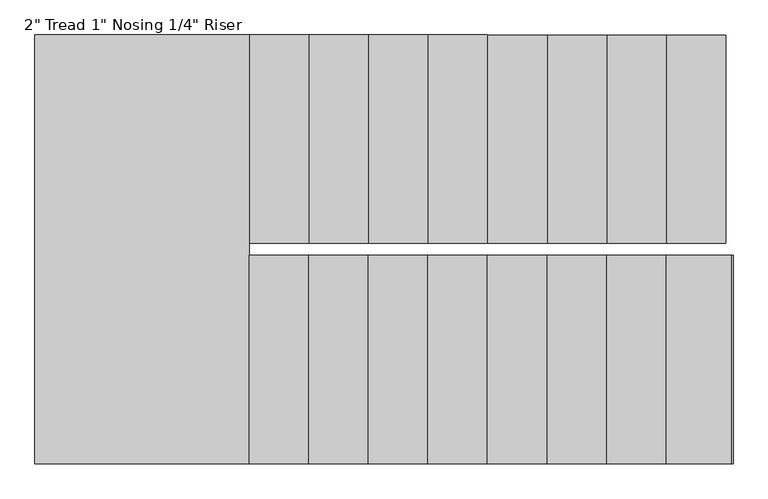
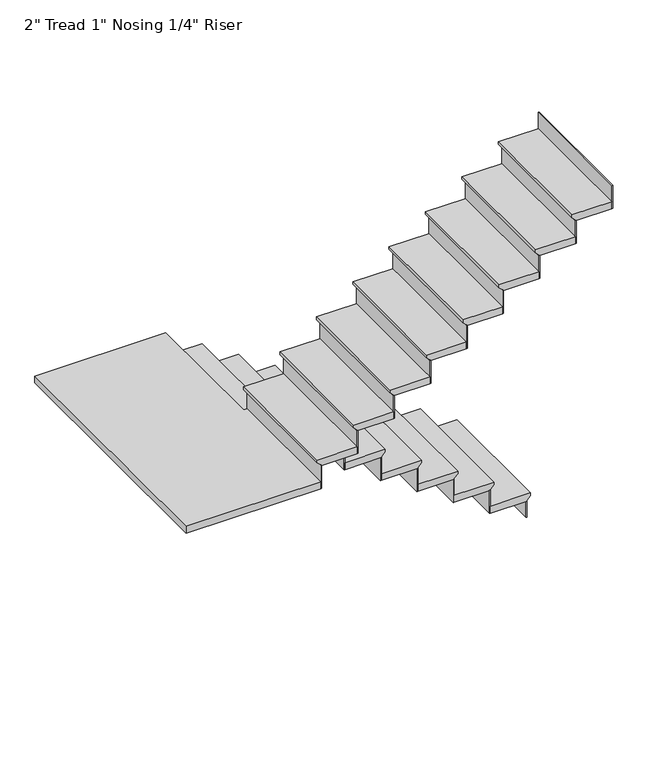
"""IFC4 building model written with IfcOpenShell, lengths in millimetres: stair flight geometry."""

from ifc_helpers import new_model, si_unit, origin, place, context, project, spatial, faceted_brep, source, transform, mapped, element, save


def stair_flight_02872950(model_context):
    return source(origin(), model_context, "Body", "Brep", [
        faceted_brep([(-2748.0012202, 5930.6309003, 6246.2833333), (-2748.0012202, 5930.6309003, 6265.3333333), (-2748.0012202, 5041.6309003, 6265.3333333), (-2748.0012202, 5041.6309003, 6246.2833333), (-2773.4012202, 5930.6309003, 6220.8833333), (-2773.4012202, 5041.6309003, 6220.8833333), (-3027.4012202, 5930.6309003, 6265.3333333), (-3027.4012202, 5041.6309003, 6265.3333333), (-2773.4012202, 5041.6309003, 6214.5333333), (-3027.4012202, 5041.6309003, 6214.5333333), (-3027.4012202, 5930.6309003, 6214.5333333), (-2773.4012202, 5930.6309003, 6214.5333333)], [[[0, 1, 2, 3]], [[4, 0, 3, 5]], [[2, 1, 6, 7]], [[8, 9, 10, 11]], [[2, 7, 9, 8, 5, 3]], [[8, 11, 4, 5]], [[6, 1, 0, 4, 11, 10]], [[7, 6, 10, 9]]]),
        faceted_brep([(-2773.4012202, 5930.6309003, 6214.5333333), (-2773.4012202, 5930.6309003, 6096.0), (-2779.7512202, 5930.6309003, 6096.0), (-2779.7512202, 5930.6309003, 6214.5333333), (-2773.4012202, 5041.6309003, 6214.5333333), (-2779.7512202, 5041.6309003, 6214.5333333), (-2779.7512202, 5041.6309003, 6096.0), (-2773.4012202, 5041.6309003, 6096.0)], [[[0, 1, 2, 3]], [[4, 5, 6, 7]], [[1, 0, 4, 7]], [[2, 1, 7, 6]], [[3, 2, 6, 5]], [[0, 3, 5, 4]]]),
        faceted_brep([(-3027.4012202, 5930.6309003, 6383.8666667), (-3027.4012202, 5930.6309003, 6214.5333333), (-3033.7512202, 5930.6309003, 6214.5333333), (-3033.7512202, 5930.6309003, 6383.8666667), (-3027.4012202, 5041.6309003, 6383.8666667), (-3033.7512202, 5041.6309003, 6383.8666667), (-3033.7512202, 5041.6309003, 6214.5333333), (-3027.4012202, 5041.6309003, 6214.5333333)], [[[0, 1, 2, 3]], [[4, 5, 6, 7]], [[1, 0, 4, 7]], [[2, 1, 7, 6]], [[3, 2, 6, 5]], [[0, 3, 5, 4]]]),
        faceted_brep([(-3002.0012202, 5041.6309003, 6434.6666667), (-3002.0012202, 5930.6309003, 6434.6666667), (-3281.4012202, 5930.6309003, 6434.6666667), (-3281.4012202, 5041.6309003, 6434.6666667), (-3027.4012202, 5041.6309003, 6383.8666667), (-3281.4012202, 5041.6309003, 6383.8666667), (-3281.4012202, 5930.6309003, 6383.8666667), (-3027.4012202, 5930.6309003, 6383.8666667), (-3027.4012202, 5041.6309003, 6390.2166667), (-3002.0012202, 5041.6309003, 6415.6166667), (-3027.4012202, 5930.6309003, 6390.2166667), (-3002.0012202, 5930.6309003, 6415.6166667)], [[[0, 1, 2, 3]], [[4, 5, 6, 7]], [[0, 3, 5, 4, 8, 9]], [[4, 7, 10, 8]], [[2, 1, 11, 10, 7, 6]], [[3, 2, 6, 5]], [[11, 1, 0, 9]], [[10, 11, 9, 8]]]),
        faceted_brep([(-3281.4012202, 5930.6309003, 6553.2), (-3281.4012202, 5930.6309003, 6383.8666667), (-3287.7512202, 5930.6309003, 6383.8666667), (-3287.7512202, 5930.6309003, 6553.2), (-3281.4012202, 5041.6309003, 6553.2), (-3287.7512202, 5041.6309003, 6553.2), (-3287.7512202, 5041.6309003, 6383.8666667), (-3281.4012202, 5041.6309003, 6383.8666667)], [[[0, 1, 2, 3]], [[4, 5, 6, 7]], [[1, 0, 4, 7]], [[2, 1, 7, 6]], [[3, 2, 6, 5]], [[0, 3, 5, 4]]]),
        faceted_brep([(-3256.0012202, 5041.6309003, 6604.0), (-3256.0012202, 5930.6309003, 6604.0), (-3535.4012202, 5930.6309003, 6604.0), (-3535.4012202, 5041.6309003, 6604.0), (-3281.4012202, 5041.6309003, 6553.2), (-3535.4012202, 5041.6309003, 6553.2), (-3535.4012202, 5930.6309003, 6553.2), (-3281.4012202, 5930.6309003, 6553.2), (-3281.4012202, 5041.6309003, 6559.55), (-3256.0012202, 5041.6309003, 6584.95), (-3281.4012202, 5930.6309003, 6559.55), (-3256.0012202, 5930.6309003, 6584.95)], [[[0, 1, 2, 3]], [[4, 5, 6, 7]], [[0, 3, 5, 4, 8, 9]], [[4, 7, 10, 8]], [[2, 1, 11, 10, 7, 6]], [[3, 2, 6, 5]], [[11, 1, 0, 9]], [[10, 11, 9, 8]]]),
        faceted_brep([(-3535.4012202, 5930.6309003, 6722.5333333), (-3535.4012202, 5930.6309003, 6553.2), (-3541.7512202, 5930.6309003, 6553.2), (-3541.7512202, 5930.6309003, 6722.5333333), (-3535.4012202, 5041.6309003, 6722.5333333), (-3541.7512202, 5041.6309003, 6722.5333333), (-3541.7512202, 5041.6309003, 6553.2), (-3535.4012202, 5041.6309003, 6553.2)], [[[0, 1, 2, 3]], [[4, 5, 6, 7]], [[1, 0, 4, 7]], [[2, 1, 7, 6]], [[3, 2, 6, 5]], [[0, 3, 5, 4]]]),
        faceted_brep([(-3510.0012202, 5041.6309003, 6773.3333333), (-3510.0012202, 5930.6309003, 6773.3333333), (-3789.4012202, 5930.6309003, 6773.3333333), (-3789.4012202, 5041.6309003, 6773.3333333), (-3535.4012202, 5041.6309003, 6722.5333333), (-3789.4012202, 5041.6309003, 6722.5333333), (-3789.4012202, 5930.6309003, 6722.5333333), (-3535.4012202, 5930.6309003, 6722.5333333), (-3535.4012202, 5041.6309003, 6728.8833333), (-3510.0012202, 5041.6309003, 6754.2833333), (-3535.4012202, 5930.6309003, 6728.8833333), (-3510.0012202, 5930.6309003, 6754.2833333)], [[[0, 1, 2, 3]], [[4, 5, 6, 7]], [[0, 3, 5, 4, 8, 9]], [[4, 7, 10, 8]], [[2, 1, 11, 10, 7, 6]], [[3, 2, 6, 5]], [[11, 1, 0, 9]], [[10, 11, 9, 8]]]),
        faceted_brep([(-3789.4012202, 5930.6309003, 6891.8666667), (-3789.4012202, 5930.6309003, 6722.5333333), (-3795.7512202, 5930.6309003, 6722.5333333), (-3795.7512202, 5930.6309003, 6891.8666667), (-3789.4012202, 5041.6309003, 6891.8666667), (-3795.7512202, 5041.6309003, 6891.8666667), (-3795.7512202, 5041.6309003, 6722.5333333), (-3789.4012202, 5041.6309003, 6722.5333333)], [[[0, 1, 2, 3]], [[4, 5, 6, 7]], [[1, 0, 4, 7]], [[2, 1, 7, 6]], [[3, 2, 6, 5]], [[0, 3, 5, 4]]]),
        faceted_brep([(-3764.0012202, 5041.6309003, 6942.6666667), (-3764.0012202, 5930.6309003, 6942.6666667), (-4043.4012202, 5930.6309003, 6942.6666667), (-4043.4012202, 5041.6309003, 6942.6666667), (-3789.4012202, 5041.6309003, 6891.8666667), (-4043.4012202, 5041.6309003, 6891.8666667), (-4043.4012202, 5930.6309003, 6891.8666667), (-3789.4012202, 5930.6309003, 6891.8666667), (-3789.4012202, 5041.6309003, 6898.2166667), (-3764.0012202, 5041.6309003, 6923.6166667), (-3789.4012202, 5930.6309003, 6898.2166667), (-3764.0012202, 5930.6309003, 6923.6166667)], [[[0, 1, 2, 3]], [[4, 5, 6, 7]], [[0, 3, 5, 4, 8, 9]], [[4, 7, 10, 8]], [[2, 1, 11, 10, 7, 6]], [[3, 2, 6, 5]], [[11, 1, 0, 9]], [[10, 11, 9, 8]]]),
        faceted_brep([(-4043.4012202, 5930.6309003, 7061.2), (-4043.4012202, 5930.6309003, 6891.8666667), (-4049.7512202, 5930.6309003, 6891.8666667), (-4049.7512202, 5930.6309003, 7061.2), (-4043.4012202, 5041.6309003, 7061.2), (-4049.7512202, 5041.6309003, 7061.2), (-4049.7512202, 5041.6309003, 6891.8666667), (-4043.4012202, 5041.6309003, 6891.8666667)], [[[0, 1, 2, 3]], [[4, 5, 6, 7]], [[1, 0, 4, 7]], [[2, 1, 7, 6]], [[3, 2, 6, 5]], [[0, 3, 5, 4]]]),
        faceted_brep([(-4018.0012202, 5041.6309003, 7112.0), (-4018.0012202, 5930.6309003, 7112.0), (-4297.4012202, 5930.6309003, 7112.0), (-4297.4012202, 5041.6309003, 7112.0), (-4043.4012202, 5041.6309003, 7061.2), (-4297.4012202, 5041.6309003, 7061.2), (-4297.4012202, 5930.6309003, 7061.2), (-4043.4012202, 5930.6309003, 7061.2), (-4043.4012202, 5041.6309003, 7067.55), (-4018.0012202, 5041.6309003, 7092.95), (-4043.4012202, 5930.6309003, 7067.55), (-4018.0012202, 5930.6309003, 7092.95)], [[[0, 1, 2, 3]], [[4, 5, 6, 7]], [[0, 3, 5, 4, 8, 9]], [[4, 7, 10, 8]], [[2, 1, 11, 10, 7, 6]], [[3, 2, 6, 5]], [[11, 1, 0, 9]], [[10, 11, 9, 8]]]),
        faceted_brep([(-4297.4012202, 5930.6309003, 7230.5333333), (-4297.4012202, 5930.6309003, 7061.2), (-4303.7512202, 5930.6309003, 7061.2), (-4303.7512202, 5930.6309003, 7230.5333333), (-4297.4012202, 5041.6309003, 7230.5333333), (-4303.7512202, 5041.6309003, 7230.5333333), (-4303.7512202, 5041.6309003, 7061.2), (-4297.4012202, 5041.6309003, 7061.2)], [[[0, 1, 2, 3]], [[4, 5, 6, 7]], [[1, 0, 4, 7]], [[2, 1, 7, 6]], [[3, 2, 6, 5]], [[0, 3, 5, 4]]]),
        faceted_brep([(-4272.0012202, 5041.6309003, 7281.3333333), (-4272.0012202, 5930.6309003, 7281.3333333), (-4551.4012202, 5930.6309003, 7281.3333333), (-4551.4012202, 5041.6309003, 7281.3333333), (-4297.4012202, 5041.6309003, 7230.5333333), (-4551.4012202, 5041.6309003, 7230.5333333), (-4551.4012202, 5930.6309003, 7230.5333333), (-4297.4012202, 5930.6309003, 7230.5333333), (-4297.4012202, 5041.6309003, 7236.8833333), (-4272.0012202, 5041.6309003, 7262.2833333), (-4297.4012202, 5930.6309003, 7236.8833333), (-4272.0012202, 5930.6309003, 7262.2833333)], [[[0, 1, 2, 3]], [[4, 5, 6, 7]], [[0, 3, 5, 4, 8, 9]], [[4, 7, 10, 8]], [[2, 1, 11, 10, 7, 6]], [[3, 2, 6, 5]], [[11, 1, 0, 9]], [[10, 11, 9, 8]]]),
        faceted_brep([(-4551.4012202, 5930.6309003, 7399.8666667), (-4551.4012202, 5930.6309003, 7230.5333333), (-4557.7512202, 5930.6309003, 7230.5333333), (-4557.7512202, 5930.6309003, 7399.8666667), (-4551.4012202, 5041.6309003, 7399.8666667), (-4557.7512202, 5041.6309003, 7399.8666667), (-4557.7512202, 5041.6309003, 7230.5333333), (-4551.4012202, 5041.6309003, 7230.5333333)], [[[0, 1, 2, 3]], [[4, 5, 6, 7]], [[1, 0, 4, 7]], [[2, 1, 7, 6]], [[3, 2, 6, 5]], [[0, 3, 5, 4]]]),
        faceted_brep([(-4526.0012202, 5041.6309003, 7450.6666667), (-4526.0012202, 5930.6309003, 7450.6666667), (-4805.4012202, 5930.6309003, 7450.6666667), (-4805.4012202, 5041.6309003, 7450.6666667), (-4551.4012202, 5041.6309003, 7399.8666667), (-4805.4012202, 5041.6309003, 7399.8666667), (-4805.4012202, 5930.6309003, 7399.8666667), (-4551.4012202, 5930.6309003, 7399.8666667), (-4551.4012202, 5041.6309003, 7406.2166667), (-4526.0012202, 5041.6309003, 7431.6166667), (-4551.4012202, 5930.6309003, 7406.2166667), (-4526.0012202, 5930.6309003, 7431.6166667)], [[[0, 1, 2, 3]], [[4, 5, 6, 7]], [[0, 3, 5, 4, 8, 9]], [[4, 7, 10, 8]], [[2, 1, 11, 10, 7, 6]], [[3, 2, 6, 5]], [[11, 1, 0, 9]], [[10, 11, 9, 8]]]),
        faceted_brep([(-4805.4012202, 5930.6309003, 7569.2), (-4805.4012202, 5930.6309003, 7399.8666667), (-4811.7512202, 5930.6309003, 7399.8666667), (-4811.7512202, 5930.6309003, 7569.2), (-4805.4012202, 5041.6309003, 7569.2), (-4811.7512202, 5041.6309003, 7569.2), (-4811.7512202, 5041.6309003, 7399.8666667), (-4805.4012202, 5041.6309003, 7399.8666667)], [[[0, 1, 2, 3]], [[4, 5, 6, 7]], [[1, 0, 4, 7]], [[2, 1, 7, 6]], [[3, 2, 6, 5]], [[0, 3, 5, 4]]]),
        faceted_brep([(-4754.6012202, 4990.8309003, 7620.0), (-4780.0012202, 4990.8309003, 7620.0), (-4780.0012202, 5930.6309003, 7620.0), (-5694.4012202, 5930.6309003, 7620.0), (-5694.4012202, 4101.8309003, 7620.0), (-4754.6012202, 4101.8309003, 7620.0), (-4780.0012202, 4990.8309003, 7569.2), (-4754.6012202, 4990.8309003, 7569.2), (-4754.6012202, 4101.8309003, 7569.2), (-5694.4012202, 4101.8309003, 7569.2), (-5694.4012202, 5930.6309003, 7569.2), (-4805.4012202, 5930.6309003, 7569.2), (-4805.4012202, 5041.6309003, 7569.2), (-4780.0012202, 5041.6309003, 7569.2), (-4780.0012202, 5041.6309003, 7600.95), (-4780.0012202, 5930.6309003, 7600.95), (-4805.4012202, 5041.6309003, 7575.55), (-4805.4012202, 5930.6309003, 7575.55)], [[[0, 1, 2, 3, 4, 5]], [[6, 7, 8, 9, 10, 11, 12, 13]], [[1, 0, 7, 6]], [[2, 1, 6, 13, 14, 15]], [[13, 12, 16, 14]], [[12, 11, 17, 16]], [[3, 2, 15, 17, 11, 10]], [[4, 3, 10, 9]], [[5, 4, 9, 8]], [[0, 5, 8, 7]], [[17, 15, 14, 16]]]),
        faceted_brep([(-4754.6012202, 4101.8309003, 7738.5333333), (-4754.6012202, 4101.8309003, 7569.2), (-4748.2512202, 4101.8309003, 7569.2), (-4748.2512202, 4101.8309003, 7738.5333333), (-4754.6012202, 4990.8309003, 7738.5333333), (-4748.2512202, 4990.8309003, 7738.5333333), (-4748.2512202, 4990.8309003, 7569.2), (-4754.6012202, 4990.8309003, 7569.2)], [[[0, 1, 2, 3]], [[4, 5, 6, 7]], [[1, 0, 4, 7]], [[2, 1, 7, 6]], [[3, 2, 6, 5]], [[0, 3, 5, 4]]]),
        faceted_brep([(-4780.0012202, 4990.8309003, 7789.3333333), (-4780.0012202, 4101.8309003, 7789.3333333), (-4500.6012202, 4101.8309003, 7789.3333333), (-4500.6012202, 4990.8309003, 7789.3333333), (-4754.6012202, 4990.8309003, 7738.5333333), (-4500.6012202, 4990.8309003, 7738.5333333), (-4500.6012202, 4101.8309003, 7738.5333333), (-4754.6012202, 4101.8309003, 7738.5333333), (-4754.6012202, 4990.8309003, 7744.8833333), (-4780.0012202, 4990.8309003, 7770.2833333), (-4754.6012202, 4101.8309003, 7744.8833333), (-4780.0012202, 4101.8309003, 7770.2833333)], [[[0, 1, 2, 3]], [[4, 5, 6, 7]], [[0, 3, 5, 4, 8, 9]], [[4, 7, 10, 8]], [[2, 1, 11, 10, 7, 6]], [[3, 2, 6, 5]], [[11, 1, 0, 9]], [[10, 11, 9, 8]]]),
        faceted_brep([(-4500.6012202, 4101.8309003, 7907.8666667), (-4500.6012202, 4101.8309003, 7738.5333333), (-4494.2512202, 4101.8309003, 7738.5333333), (-4494.2512202, 4101.8309003, 7907.8666667), (-4500.6012202, 4990.8309003, 7907.8666667), (-4494.2512202, 4990.8309003, 7907.8666667), (-4494.2512202, 4990.8309003, 7738.5333333), (-4500.6012202, 4990.8309003, 7738.5333333)], [[[0, 1, 2, 3]], [[4, 5, 6, 7]], [[1, 0, 4, 7]], [[2, 1, 7, 6]], [[3, 2, 6, 5]], [[0, 3, 5, 4]]]),
        faceted_brep([(-4526.0012202, 4990.8309003, 7958.6666667), (-4526.0012202, 4101.8309003, 7958.6666667), (-4246.6012202, 4101.8309003, 7958.6666667), (-4246.6012202, 4990.8309003, 7958.6666667), (-4500.6012202, 4990.8309003, 7907.8666667), (-4246.6012202, 4990.8309003, 7907.8666667), (-4246.6012202, 4101.8309003, 7907.8666667), (-4500.6012202, 4101.8309003, 7907.8666667), (-4500.6012202, 4990.8309003, 7914.2166667), (-4526.0012202, 4990.8309003, 7939.6166667), (-4500.6012202, 4101.8309003, 7914.2166667), (-4526.0012202, 4101.8309003, 7939.6166667)], [[[0, 1, 2, 3]], [[4, 5, 6, 7]], [[0, 3, 5, 4, 8, 9]], [[4, 7, 10, 8]], [[2, 1, 11, 10, 7, 6]], [[3, 2, 6, 5]], [[11, 1, 0, 9]], [[10, 11, 9, 8]]]),
        faceted_brep([(-4246.6012202, 4101.8309003, 8077.2), (-4246.6012202, 4101.8309003, 7907.8666667), (-4240.2512202, 4101.8309003, 7907.8666667), (-4240.2512202, 4101.8309003, 8077.2), (-4246.6012202, 4990.8309003, 8077.2), (-4240.2512202, 4990.8309003, 8077.2), (-4240.2512202, 4990.8309003, 7907.8666667), (-4246.6012202, 4990.8309003, 7907.8666667)], [[[0, 1, 2, 3]], [[4, 5, 6, 7]], [[1, 0, 4, 7]], [[2, 1, 7, 6]], [[3, 2, 6, 5]], [[0, 3, 5, 4]]]),
        faceted_brep([(-4272.0012202, 4990.8309003, 8128.0), (-4272.0012202, 4101.8309003, 8128.0), (-3992.6012202, 4101.8309003, 8128.0), (-3992.6012202, 4990.8309003, 8128.0), (-4246.6012202, 4990.8309003, 8077.2), (-3992.6012202, 4990.8309003, 8077.2), (-3992.6012202, 4101.8309003, 8077.2), (-4246.6012202, 4101.8309003, 8077.2), (-4246.6012202, 4990.8309003, 8083.55), (-4272.0012202, 4990.8309003, 8108.95), (-4246.6012202, 4101.8309003, 8083.55), (-4272.0012202, 4101.8309003, 8108.95)], [[[0, 1, 2, 3]], [[4, 5, 6, 7]], [[0, 3, 5, 4, 8, 9]], [[4, 7, 10, 8]], [[2, 1, 11, 10, 7, 6]], [[3, 2, 6, 5]], [[11, 1, 0, 9]], [[10, 11, 9, 8]]]),
        faceted_brep([(-3992.6012202, 4101.8309003, 8246.5333333), (-3992.6012202, 4101.8309003, 8077.2), (-3986.2512202, 4101.8309003, 8077.2), (-3986.2512202, 4101.8309003, 8246.5333333), (-3992.6012202, 4990.8309003, 8246.5333333), (-3986.2512202, 4990.8309003, 8246.5333333), (-3986.2512202, 4990.8309003, 8077.2), (-3992.6012202, 4990.8309003, 8077.2)], [[[0, 1, 2, 3]], [[4, 5, 6, 7]], [[1, 0, 4, 7]], [[2, 1, 7, 6]], [[3, 2, 6, 5]], [[0, 3, 5, 4]]]),
        faceted_brep([(-4018.0012202, 4990.8309003, 8297.3333333), (-4018.0012202, 4101.8309003, 8297.3333333), (-3738.6012202, 4101.8309003, 8297.3333333), (-3738.6012202, 4990.8309003, 8297.3333333), (-3992.6012202, 4990.8309003, 8246.5333333), (-3738.6012202, 4990.8309003, 8246.5333333), (-3738.6012202, 4101.8309003, 8246.5333333), (-3992.6012202, 4101.8309003, 8246.5333333), (-3992.6012202, 4990.8309003, 8252.8833333), (-4018.0012202, 4990.8309003, 8278.2833333), (-3992.6012202, 4101.8309003, 8252.8833333), (-4018.0012202, 4101.8309003, 8278.2833333)], [[[0, 1, 2, 3]], [[4, 5, 6, 7]], [[0, 3, 5, 4, 8, 9]], [[4, 7, 10, 8]], [[2, 1, 11, 10, 7, 6]], [[3, 2, 6, 5]], [[11, 1, 0, 9]], [[10, 11, 9, 8]]]),
        faceted_brep([(-3738.6012202, 4101.8309003, 8415.8666667), (-3738.6012202, 4101.8309003, 8246.5333333), (-3732.2512202, 4101.8309003, 8246.5333333), (-3732.2512202, 4101.8309003, 8415.8666667), (-3738.6012202, 4990.8309003, 8415.8666667), (-3732.2512202, 4990.8309003, 8415.8666667), (-3732.2512202, 4990.8309003, 8246.5333333), (-3738.6012202, 4990.8309003, 8246.5333333)], [[[0, 1, 2, 3]], [[4, 5, 6, 7]], [[1, 0, 4, 7]], [[2, 1, 7, 6]], [[3, 2, 6, 5]], [[0, 3, 5, 4]]]),
        faceted_brep([(-3764.0012202, 4990.8309003, 8466.6666667), (-3764.0012202, 4101.8309003, 8466.6666667), (-3484.6012202, 4101.8309003, 8466.6666667), (-3484.6012202, 4990.8309003, 8466.6666667), (-3738.6012202, 4990.8309003, 8415.8666667), (-3484.6012202, 4990.8309003, 8415.8666667), (-3484.6012202, 4101.8309003, 8415.8666667), (-3738.6012202, 4101.8309003, 8415.8666667), (-3738.6012202, 4990.8309003, 8422.2166667), (-3764.0012202, 4990.8309003, 8447.6166667), (-3738.6012202, 4101.8309003, 8422.2166667), (-3764.0012202, 4101.8309003, 8447.6166667)], [[[0, 1, 2, 3]], [[4, 5, 6, 7]], [[0, 3, 5, 4, 8, 9]], [[4, 7, 10, 8]], [[2, 1, 11, 10, 7, 6]], [[3, 2, 6, 5]], [[11, 1, 0, 9]], [[10, 11, 9, 8]]]),
        faceted_brep([(-3484.6012202, 4101.8309003, 8585.2), (-3484.6012202, 4101.8309003, 8415.8666667), (-3478.2512202, 4101.8309003, 8415.8666667), (-3478.2512202, 4101.8309003, 8585.2), (-3484.6012202, 4990.8309003, 8585.2), (-3478.2512202, 4990.8309003, 8585.2), (-3478.2512202, 4990.8309003, 8415.8666667), (-3484.6012202, 4990.8309003, 8415.8666667)], [[[0, 1, 2, 3]], [[4, 5, 6, 7]], [[1, 0, 4, 7]], [[2, 1, 7, 6]], [[3, 2, 6, 5]], [[0, 3, 5, 4]]]),
        faceted_brep([(-3510.0012202, 4990.8309003, 8636.0), (-3510.0012202, 4101.8309003, 8636.0), (-3230.6012202, 4101.8309003, 8636.0), (-3230.6012202, 4990.8309003, 8636.0), (-3484.6012202, 4990.8309003, 8585.2), (-3230.6012202, 4990.8309003, 8585.2), (-3230.6012202, 4101.8309003, 8585.2), (-3484.6012202, 4101.8309003, 8585.2), (-3484.6012202, 4990.8309003, 8591.55), (-3510.0012202, 4990.8309003, 8616.95), (-3484.6012202, 4101.8309003, 8591.55), (-3510.0012202, 4101.8309003, 8616.95)], [[[0, 1, 2, 3]], [[4, 5, 6, 7]], [[0, 3, 5, 4, 8, 9]], [[4, 7, 10, 8]], [[2, 1, 11, 10, 7, 6]], [[3, 2, 6, 5]], [[11, 1, 0, 9]], [[10, 11, 9, 8]]]),
        faceted_brep([(-3230.6012202, 4101.8309003, 8754.5333333), (-3230.6012202, 4101.8309003, 8585.2), (-3224.2512202, 4101.8309003, 8585.2), (-3224.2512202, 4101.8309003, 8754.5333333), (-3230.6012202, 4990.8309003, 8754.5333333), (-3224.2512202, 4990.8309003, 8754.5333333), (-3224.2512202, 4990.8309003, 8585.2), (-3230.6012202, 4990.8309003, 8585.2)], [[[0, 1, 2, 3]], [[4, 5, 6, 7]], [[1, 0, 4, 7]], [[2, 1, 7, 6]], [[3, 2, 6, 5]], [[0, 3, 5, 4]]]),
        faceted_brep([(-3256.0012202, 4990.8309003, 8805.3333333), (-3256.0012202, 4101.8309003, 8805.3333333), (-2976.6012202, 4101.8309003, 8805.3333333), (-2976.6012202, 4990.8309003, 8805.3333333), (-3230.6012202, 4990.8309003, 8754.5333333), (-2976.6012202, 4990.8309003, 8754.5333333), (-2976.6012202, 4101.8309003, 8754.5333333), (-3230.6012202, 4101.8309003, 8754.5333333), (-3230.6012202, 4990.8309003, 8760.8833333), (-3256.0012202, 4990.8309003, 8786.2833333), (-3230.6012202, 4101.8309003, 8760.8833333), (-3256.0012202, 4101.8309003, 8786.2833333)], [[[0, 1, 2, 3]], [[4, 5, 6, 7]], [[0, 3, 5, 4, 8, 9]], [[4, 7, 10, 8]], [[2, 1, 11, 10, 7, 6]], [[3, 2, 6, 5]], [[11, 1, 0, 9]], [[10, 11, 9, 8]]]),
        faceted_brep([(-2976.6012202, 4101.8309003, 8923.8666667), (-2976.6012202, 4101.8309003, 8754.5333333), (-2970.2512202, 4101.8309003, 8754.5333333), (-2970.2512202, 4101.8309003, 8923.8666667), (-2976.6012202, 4990.8309003, 8923.8666667), (-2970.2512202, 4990.8309003, 8923.8666667), (-2970.2512202, 4990.8309003, 8754.5333333), (-2976.6012202, 4990.8309003, 8754.5333333)], [[[0, 1, 2, 3]], [[4, 5, 6, 7]], [[1, 0, 4, 7]], [[2, 1, 7, 6]], [[3, 2, 6, 5]], [[0, 3, 5, 4]]]),
        faceted_brep([(-2722.6012202, 4101.8309003, 9093.2), (-2722.6012202, 4101.8309003, 8923.8666667), (-2716.2512202, 4101.8309003, 8923.8666667), (-2716.2512202, 4101.8309003, 9093.2), (-2722.6012202, 4990.8309003, 9093.2), (-2716.2512202, 4990.8309003, 9093.2), (-2716.2512202, 4990.8309003, 8923.8666667), (-2722.6012202, 4990.8309003, 8923.8666667)], [[[0, 1, 2, 3]], [[4, 5, 6, 7]], [[1, 0, 4, 7]], [[2, 1, 7, 6]], [[3, 2, 6, 5]], [[0, 3, 5, 4]]]),
        faceted_brep([(-3002.0012202, 4990.8309003, 8974.6666667), (-3002.0012202, 4101.8309003, 8974.6666667), (-2722.6012202, 4101.8309003, 8974.6666667), (-2722.6012202, 4990.8309003, 8974.6666667), (-2976.6012202, 4990.8309003, 8923.8666667), (-2722.6012202, 4990.8309003, 8923.8666667), (-2722.6012202, 4101.8309003, 8923.8666667), (-2976.6012202, 4101.8309003, 8923.8666667), (-2976.6012202, 4990.8309003, 8930.2166667), (-3002.0012202, 4990.8309003, 8955.6166667), (-2976.6012202, 4101.8309003, 8930.2166667), (-3002.0012202, 4101.8309003, 8955.6166667)], [[[0, 1, 2, 3]], [[4, 5, 6, 7]], [[0, 3, 5, 4, 8, 9]], [[4, 7, 10, 8]], [[2, 1, 11, 10, 7, 6]], [[3, 2, 6, 5]], [[11, 1, 0, 9]], [[10, 11, 9, 8]]]),
    ])


if __name__ == "__main__":
    model = new_model("IFC4")
    model_context = context("Model", 3, world=origin())
    ifc_project = project(units=[si_unit("LENGTHUNIT", "METRE", prefix="MILLI")], contexts=[model_context])
    site = spatial("IfcSite", under=ifc_project)
    building = spatial("IfcBuilding", under=site)
    placement = place(None, origin())
    stair_flight_shape = stair_flight_02872950(model_context)
    element("IfcStairFlight", 1, ObjectType="2\" Tread 1\" Nosing 1/4\" Riser", at=placement, inside=building, context=model_context, shape_type="MappedRepresentation", body=[
        mapped(stair_flight_shape, transform((0.0, 0.0, 0.0), x_axis=(1.0, 0.0, 0.0), y_axis=(0.0, 1.0, 0.0), z_axis=(0.0, 0.0, 1.0))),
    ])
    save(model, "model.ifc")
